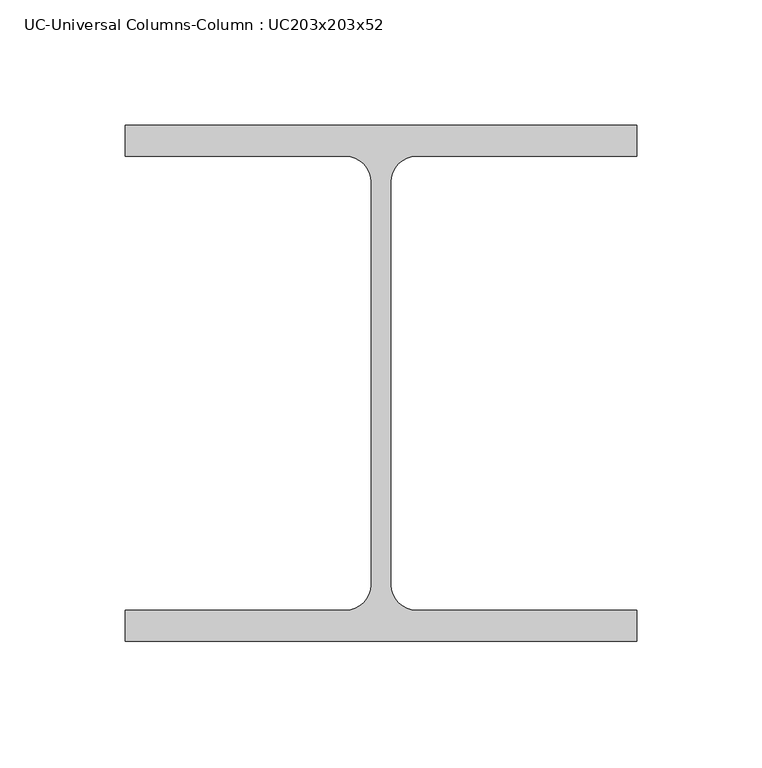
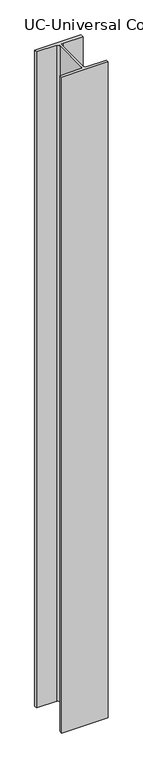
"""IFC4 building model written with IfcOpenShell, lengths in millimetres: column geometry, UC-Universal Columns-Column : UC203x203x52."""

from ifc_helpers import new_model, si_unit, point, frame, frame_2d, origin, place, context, project, spatial, polyline, circle_curve, trimmed, segment, composite_curve, outline, extrude, source, transform, mapped, element, save


def uc_universal_columns_column_uc203x203x52_01cb6b5e(model_context):
    return source(origin(), model_context, "Body", "SweptSolid", [
        extrude(outline(composite_curve([segment(polyline([(102.15, 103.1), (102.15, 90.6), (14.15, 90.6)]), True, "CONTINUOUS"), segment(trimmed(circle_curve(frame_2d((14.15, 80.4)), 10.2), [point((14.15, 90.6))], [point((3.95, 80.4))], True, "CARTESIAN"), True, "CONTINUOUS"), segment(polyline([(3.95, 80.4), (3.95, -80.4)]), True, "CONTINUOUS"), segment(trimmed(circle_curve(frame_2d((14.15, -80.4)), 10.2), [point((3.95, -80.4))], [point((14.15, -90.6))], True, "CARTESIAN"), True, "CONTINUOUS"), segment(polyline([(14.15, -90.6), (102.15, -90.6), (102.15, -103.1), (-102.15, -103.1), (-102.15, -90.6), (-14.15, -90.6)]), True, "CONTINUOUS"), segment(trimmed(circle_curve(frame_2d((-14.15, -80.4)), 10.2), [point((-14.15, -90.6))], [point((-3.95, -80.4))], True, "CARTESIAN"), True, "CONTINUOUS"), segment(polyline([(-3.95, -80.4), (-3.95, 80.4)]), True, "CONTINUOUS"), segment(trimmed(circle_curve(frame_2d((-14.15, 80.4)), 10.2), [point((-3.95, 80.4))], [point((-14.15, 90.6))], True, "CARTESIAN"), True, "CONTINUOUS"), segment(polyline([(-14.15, 90.6), (-102.15, 90.6), (-102.15, 103.1), (102.15, 103.1)]), True, "CONTINUOUS")], self_intersect=False)), frame((0.0, 0.0, 6096.0), z_axis=(0.0, 0.0, 1.0), x_axis=(1.0, 0.0, 0.0)), (0.0, 0.0, 1.0), 3048.0),
    ])


if __name__ == "__main__":
    model = new_model("IFC4")
    model_context = context("Model", 3, world=origin())
    ifc_project = project(units=[si_unit("LENGTHUNIT", "METRE", prefix="MILLI")], contexts=[model_context])
    site = spatial("IfcSite", under=ifc_project)
    building = spatial("IfcBuilding", under=site)
    placement = place(None, origin())
    uc_universal_columns_column_uc203x203x52_shape = uc_universal_columns_column_uc203x203x52_01cb6b5e(model_context)
    element("IfcColumn", 1, ObjectType="UC-Universal Columns-Column : UC203x203x52", at=placement, inside=building, context=model_context, shape_type="MappedRepresentation", body=[
        mapped(uc_universal_columns_column_uc203x203x52_shape, transform((0.0, 0.0, 0.0), x_axis=(1.0, 0.0, 0.0), y_axis=(0.0, 1.0, 0.0), z_axis=(0.0, 0.0, 1.0))),
    ])
    save(model, "model.ifc")

# Revit data of these elements
# Type "UC-Universal Columns-Column : UC203x203x52"
#   Section Name Key = "UC203x203x52"
#   Width = 20.43 cm
#   Web Thickness = 0.79 cm
#   Web Fillet = 1.02 cm
#   Warping Constant = 167000.0 cm⁶
#   Torsional Moment of Inertia = 31.80 cm⁴
#   Section Area = 66.0 cm²
#   Plastic Modulus weak axis = 264.0 cm³
#   Plastic Modulus strong axis = 567.0 cm³
#   Nominal Weight = 51.9998 kgf/m
#   Moment of Inertia weak axis = 1778.00 cm⁴
#   Moment of Inertia strong axis = 5259.00 cm⁴
#   Height = 20.62 cm
#   Flange Thickness = 1.25 cm
#   Elastic Modulus weak axis = 174.0 cm³
#   Elastic Modulus strong axis = 510.0 cm³
#   Centroid Vertical = 10.31 cm
#   Centroid Horizontal = 10.215 cm
#   Bolt Spacing = 14.0 cm
#   Structural Material [instance default] = Metal - Steel 43-275
#   Type Comments = ""
#   Assembly Code = ""
# Element 1 (IfcColumn, "UC-Universal Columns-Column : UC203x203x52")
#   Materials on its faces: "Metal - Steel 43-275"
# Materials
#   "Metal - Steel 43-275": class "Metal", colour RGB 247 247 247, transparency 0, Cost = 0
